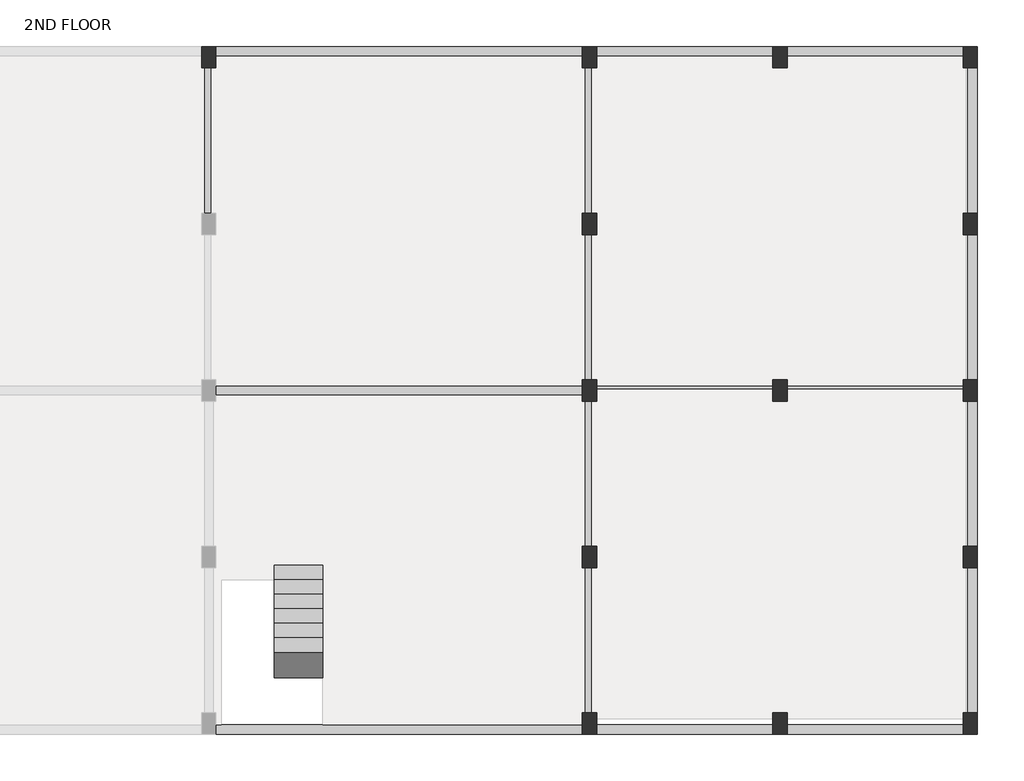
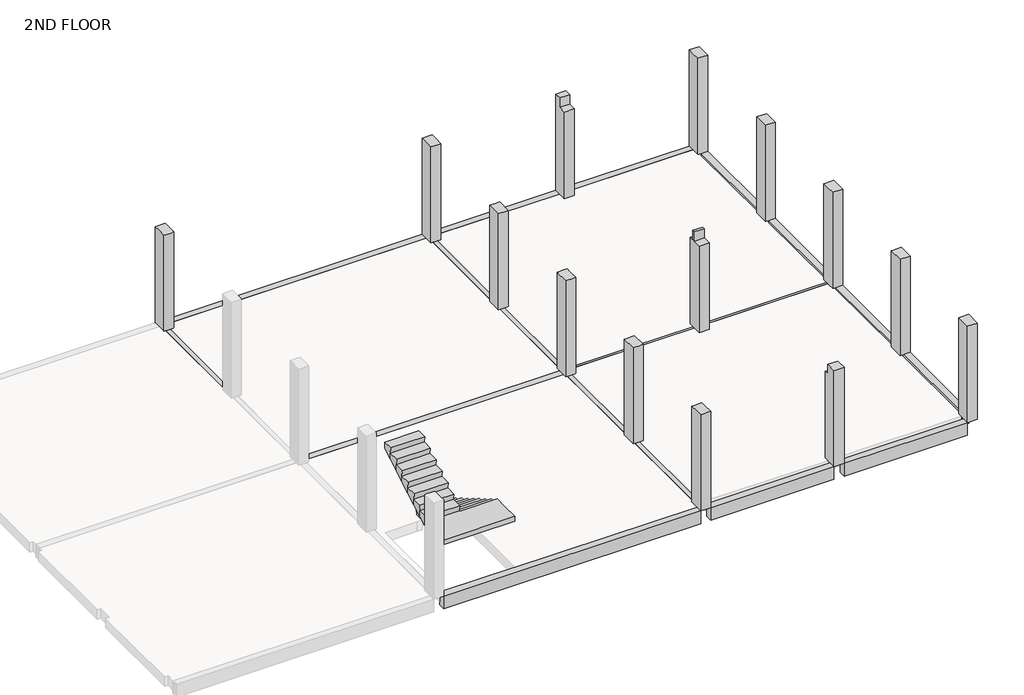
# One storey, part 2 of 2: 18 beams, 14 columns, 1 stair flight.
"""IFC4 building model written with IfcOpenShell, lengths in millimetres."""

from ifc_helpers import new_model, si_unit, frame, origin, place, context, project, spatial, polyline, outline, extrude, faceted_brep, element, save

model = new_model("IFC4")

# Units and contexts
model_context = context("Model", 3, world=origin())
ifc_project = project(units=[si_unit("LENGTHUNIT", "METRE", prefix="MILLI")], contexts=[model_context])

# Site, building, storey
site = spatial("IfcSite", under=ifc_project)
building = spatial("IfcBuilding", under=site)
storey = spatial("IfcBuildingStorey", under=building, Name="2ND FLOOR", Elevation=6096.0)

# Beams
placement = place(None, origin())
element("IfcBeam", 1, ObjectType="M_Concrete-Rectangular Beam : 200MMX400MM", at=placement, inside=storey, context=model_context, shape_type="Brep", body=[
    faceted_brep([(4019.3125983, 15797.7008557, 6096.0), (4019.3125983, 15997.7008557, 6096.0), (-3680.6874017, 15997.7008557, 6096.0), (-3680.6874017, 15797.7008557, 6096.0), (4019.3125983, 15797.7008557, 5696.0), (4019.3125983, 15797.7008557, 5796.0), (-3680.6874017, 15797.7008557, 5796.0), (-3680.6874017, 15797.7008557, 5696.0), (4019.3125983, 15997.7008557, 5696.0), (-3680.6874017, 15997.7008557, 5696.0)], [[[0, 1, 2, 3]], [[4, 5, 0, 3, 6, 7]], [[8, 4, 7, 9]], [[1, 8, 9, 2]], [[1, 0, 5, 4, 8]], [[2, 9, 7, 6, 3]]]),
])
element("IfcBeam", 2, ObjectType="M_Concrete-Rectangular Beam : 200MMX400MM", at=placement, inside=storey, context=model_context, shape_type="Brep", body=[
    faceted_brep([(8019.3125983, 15797.7008557, 6096.0), (8019.3125983, 15997.7008557, 6096.0), (4319.3125983, 15997.7008557, 6096.0), (4319.3125983, 15797.7008557, 6096.0), (8019.3125983, 15797.7008557, 5696.0), (4319.3125983, 15797.7008557, 5796.0), (4319.3125983, 15797.7008557, 5696.0), (8019.3125983, 15997.7008557, 5696.0), (4319.3125983, 15997.7008557, 5696.0)], [[[0, 1, 2, 3]], [[4, 0, 3, 5, 6]], [[7, 4, 6, 8]], [[1, 7, 8, 2]], [[2, 8, 6, 5, 3]], [[1, 0, 4, 7]]]),
])
element("IfcBeam", 3, ObjectType="M_Concrete-Rectangular Beam : 200MMX400MM", at=placement, inside=storey, context=model_context, shape_type="Brep", body=[
    faceted_brep([(12019.3125983, 15797.7008557, 6096.0), (12019.3125983, 15997.7008557, 6096.0), (8319.3125983, 15997.7008557, 6096.0), (8319.3125983, 15797.7008557, 6096.0), (12019.3125983, 15797.7008557, 5696.0), (12019.3125983, 15797.7008557, 5796.0), (8319.3125983, 15797.7008557, 5696.0), (12019.3125983, 15997.7008557, 5696.0), (8319.3125983, 15997.7008557, 5696.0)], [[[0, 1, 2, 3]], [[4, 5, 0, 3, 6]], [[7, 4, 6, 8]], [[1, 7, 8, 2]], [[2, 8, 6, 3]], [[1, 0, 5, 4, 7]]]),
])
element("IfcBeam", 4, ObjectType="M_Concrete-Rectangular Beam : 200MMX400MM", at=placement, inside=storey, context=model_context, shape_type="SweptSolid", body=[
    extrude(outline(polyline([(12319.3125983, 12497.7008557), (12119.3125983, 12497.7008557), (12119.3125983, 15547.7008557), (12319.3125983, 15547.7008557), (12319.3125983, 12497.7008557)])), frame((0.0, 0.0, 5696.0), z_axis=(0.0, 0.0, 1.0), x_axis=(1.0, 0.0, 0.0)), (0.0, 0.0, 1.0), 400.0),
])
element("IfcBeam", 5, ObjectType="M_Concrete-Rectangular Beam : 200MMX400MM", at=placement, inside=storey, context=model_context, shape_type="SweptSolid", body=[
    extrude(outline(polyline([(12319.3125983, 1997.7008557), (12119.3125983, 1997.7008557), (12119.3125983, 5047.7008557), (12319.3125983, 5047.7008557), (12319.3125983, 1997.7008557)])), frame((0.0, 0.0, 5696.0), z_axis=(0.0, 0.0, 1.0), x_axis=(1.0, 0.0, 0.0)), (0.0, 0.0, 1.0), 400.0),
])
element("IfcBeam", 6, ObjectType="M_Concrete-Rectangular Beam : 200MMX400MM", at=placement, inside=storey, context=model_context, shape_type="SweptSolid", body=[
    extrude(outline(polyline([(8319.3125983, 1547.7008557), (8319.3125983, 1747.7008557), (12019.3125983, 1747.7008557), (12019.3125983, 1547.7008557), (8319.3125983, 1547.7008557)])), frame((0.0, 0.0, 5696.0), z_axis=(0.0, 0.0, 1.0), x_axis=(1.0, 0.0, 0.0)), (0.0, 0.0, 1.0), 400.0),
])
element("IfcBeam", 7, ObjectType="M_Concrete-Rectangular Beam : 200MMX400MM", at=placement, inside=storey, context=model_context, shape_type="SweptSolid", body=[
    extrude(outline(polyline([(8019.3125983, 1747.7008557), (8019.3125983, 1547.7008557), (4319.3125983, 1547.7008557), (4319.3125983, 1747.7008557), (8019.3125983, 1747.7008557)])), frame((0.0, 0.0, 5696.0), z_axis=(0.0, 0.0, 1.0), x_axis=(1.0, 0.0, 0.0)), (0.0, 0.0, 1.0), 400.0),
])
element("IfcBeam", 8, ObjectType="M_Concrete-Rectangular Beam : 200MMX400MM", at=placement, inside=storey, context=model_context, shape_type="Brep", body=[
    faceted_brep([(-3680.6874017, 1747.7008557, 6096.0), (-3680.6874017, 1547.7008557, 6096.0), (4019.3125983, 1547.7008557, 6096.0), (4019.3125983, 1747.7008557, 6096.0), (-1437.0874017, 1747.7008557, 6096.0), (-3570.6874017, 1747.7008557, 6096.0), (-3680.6874017, 1747.7008557, 5696.0), (-3680.6874017, 1747.7008557, 5796.0), (4019.3125983, 1747.7008557, 5796.0), (4019.3125983, 1747.7008557, 5696.0), (-3680.6874017, 1547.7008557, 5696.0), (4019.3125983, 1547.7008557, 5696.0)], [[[0, 1, 2, 3, 4, 5]], [[6, 7, 0, 5, 4, 3, 8, 9]], [[10, 6, 9, 11]], [[1, 10, 11, 2]], [[1, 0, 7, 6, 10]], [[2, 11, 9, 8, 3]]]),
])
element("IfcBeam", 9, ObjectType="M_Concrete-Rectangular Beam : 200MMX400MM", at=placement, inside=storey, context=model_context, shape_type="Brep", body=[
    faceted_brep([(4019.3125983, 8872.7008557, 6096.0), (-3680.6874017, 8872.7008557, 6096.0), (-3680.6874017, 8672.7008557, 6096.0), (4019.3125983, 8672.7008557, 6096.0), (-3680.6874017, 8672.7008557, 5796.0), (-3680.6874017, 8672.7008557, 5696.0), (4019.3125983, 8672.7008557, 5696.0), (4019.3125983, 8672.7008557, 5796.0), (-3680.6874017, 8872.7008557, 5696.0), (4019.3125983, 8872.7008557, 5696.0), (4019.3125983, 8872.7008557, 5796.0), (-3680.6874017, 8872.7008557, 5796.0)], [[[0, 1, 2, 3]], [[3, 2, 4, 5, 6, 7]], [[6, 5, 8, 9]], [[1, 0, 10, 9, 8, 11]], [[8, 5, 4, 2, 1, 11]], [[0, 3, 7, 6, 9, 10]]]),
])
element("IfcBeam", 10, ObjectType="M_Concrete-Rectangular Beam : 200MMX400MM", at=placement, inside=storey, context=model_context, shape_type="Brep", body=[
    faceted_brep([(8019.3125983, 8872.7008557, 6096.0), (4319.3125983, 8872.7008557, 6096.0), (4319.3125983, 8797.7008557, 6096.0), (8019.3125983, 8797.7008557, 6096.0), (4319.3125983, 8672.7008557, 5696.0), (8019.3125983, 8672.7008557, 5696.0), (8019.3125983, 8672.7008557, 5796.0), (4319.3125983, 8672.7008557, 5796.0), (4319.3125983, 8872.7008557, 5696.0), (8019.3125983, 8872.7008557, 5696.0), (8019.3125983, 8872.7008557, 5796.0), (4319.3125983, 8872.7008557, 5796.0), (4319.3125983, 8797.7008557, 5796.0), (8019.3125983, 8797.7008557, 5796.0)], [[[0, 1, 2, 3]], [[4, 5, 6, 7]], [[5, 4, 8, 9]], [[1, 0, 10, 9, 8, 11]], [[8, 4, 7, 12, 2, 1, 11]], [[5, 9, 10, 0, 3, 13, 6]], [[13, 12, 7, 6]], [[12, 13, 3, 2]]]),
])
element("IfcBeam", 11, ObjectType="M_Concrete-Rectangular Beam : 200MMX400MM", at=placement, inside=storey, context=model_context, shape_type="Brep", body=[
    faceted_brep([(12019.3125983, 8872.7008557, 6096.0), (8319.3125983, 8872.7008557, 6096.0), (8319.3125983, 8797.7008557, 6096.0), (12019.3125983, 8797.7008557, 6096.0), (8319.3125983, 8672.7008557, 5696.0), (12019.3125983, 8672.7008557, 5696.0), (12019.3125983, 8672.7008557, 5796.0), (8319.3125983, 8672.7008557, 5796.0), (8319.3125983, 8872.7008557, 5696.0), (12019.3125983, 8872.7008557, 5696.0), (12019.3125983, 8872.7008557, 5796.0), (8319.3125983, 8872.7008557, 5796.0), (12019.3125983, 8797.7008557, 5796.0), (8319.3125983, 8797.7008557, 5796.0)], [[[0, 1, 2, 3]], [[4, 5, 6, 7]], [[5, 4, 8, 9]], [[1, 0, 10, 9, 8, 11]], [[5, 9, 10, 0, 3, 12, 6]], [[8, 4, 7, 13, 2, 1, 11]], [[12, 13, 7, 6]], [[13, 12, 3, 2]]]),
])
element("IfcBeam", 12, ObjectType="M_Concrete-Rectangular Beam : 200MMX400MM", at=placement, inside=storey, context=model_context, shape_type="SweptSolid", body=[
    extrude(outline(polyline([(12319.3125983, 5497.7008557), (12119.3125983, 5497.7008557), (12119.3125983, 8547.7008557), (12319.3125983, 8547.7008557), (12319.3125983, 5497.7008557)])), frame((0.0, 0.0, 5696.0), z_axis=(0.0, 0.0, 1.0), x_axis=(1.0, 0.0, 0.0)), (0.0, 0.0, 1.0), 400.0),
])
element("IfcBeam", 13, ObjectType="M_Concrete-Rectangular Beam : 200MMX400MM", at=placement, inside=storey, context=model_context, shape_type="SweptSolid", body=[
    extrude(outline(polyline([(12119.3125983, 12047.7008557), (12319.3125983, 12047.7008557), (12319.3125983, 8997.7008557), (12119.3125983, 8997.7008557), (12119.3125983, 12047.7008557)])), frame((0.0, 0.0, 5696.0), z_axis=(0.0, 0.0, 1.0), x_axis=(1.0, 0.0, 0.0)), (0.0, 0.0, 1.0), 400.0),
])
element("IfcBeam", 14, ObjectType="M_Concrete-Rectangular Beam : 200MMX400MM", at=placement, inside=storey, context=model_context, shape_type="Brep", body=[
    faceted_brep([(4069.3125983, 5047.7008557, 6096.0), (4069.3125983, 1997.7008557, 6096.0), (4219.3125983, 1997.7008557, 6096.0), (4219.3125983, 5047.7008557, 6096.0), (4269.3125983, 1997.7008557, 5696.0), (4269.3125983, 5047.7008557, 5696.0), (4269.3125983, 5047.7008557, 5796.0), (4269.3125983, 1997.7008557, 5796.0), (4069.3125983, 1997.7008557, 5696.0), (4069.3125983, 5047.7008557, 5696.0), (4069.3125983, 5047.7008557, 5796.0), (4069.3125983, 1997.7008557, 5796.0), (4219.3125983, 1997.7008557, 5796.0), (4219.3125983, 5047.7008557, 5796.0)], [[[0, 1, 2, 3]], [[4, 5, 6, 7]], [[5, 4, 8, 9]], [[1, 0, 10, 9, 8, 11]], [[8, 4, 7, 12, 2, 1, 11]], [[5, 9, 10, 0, 3, 13, 6]], [[13, 12, 7, 6]], [[12, 13, 3, 2]]]),
])
element("IfcBeam", 15, ObjectType="M_Concrete-Rectangular Beam : 200MMX400MM", at=placement, inside=storey, context=model_context, shape_type="Brep", body=[
    faceted_brep([(4069.3125983, 8547.7008557, 6096.0), (4069.3125983, 5497.7008557, 6096.0), (4219.3125983, 5497.7008557, 6096.0), (4219.3125983, 8547.7008557, 6096.0), (4269.3125983, 5497.7008557, 5696.0), (4269.3125983, 8547.7008557, 5696.0), (4269.3125983, 8547.7008557, 5796.0), (4269.3125983, 5497.7008557, 5796.0), (4069.3125983, 5497.7008557, 5696.0), (4069.3125983, 8547.7008557, 5696.0), (4069.3125983, 8547.7008557, 5796.0), (4069.3125983, 5497.7008557, 5796.0), (4219.3125983, 8547.7008557, 5796.0), (4219.3125983, 5497.7008557, 5796.0)], [[[0, 1, 2, 3]], [[4, 5, 6, 7]], [[5, 4, 8, 9]], [[1, 0, 10, 9, 8, 11]], [[5, 9, 10, 0, 3, 12, 6]], [[8, 4, 7, 13, 2, 1, 11]], [[12, 13, 7, 6]], [[13, 12, 3, 2]]]),
])
element("IfcBeam", 16, ObjectType="M_Concrete-Rectangular Beam : 200MMX400MM", at=placement, inside=storey, context=model_context, shape_type="Brep", body=[
    faceted_brep([(4069.3125983, 12047.7008557, 6096.0), (4069.3125983, 8997.7008557, 6096.0), (4219.3125983, 8997.7008557, 6096.0), (4219.3125983, 12047.7008557, 6096.0), (4269.3125983, 8997.7008557, 5696.0), (4269.3125983, 12047.7008557, 5696.0), (4269.3125983, 12047.7008557, 5796.0), (4269.3125983, 8997.7008557, 5796.0), (4069.3125983, 8997.7008557, 5696.0), (4069.3125983, 12047.7008557, 5696.0), (4069.3125983, 12047.7008557, 5796.0), (4069.3125983, 8997.7008557, 5796.0), (4219.3125983, 8997.7008557, 5796.0), (4219.3125983, 12047.7008557, 5796.0)], [[[0, 1, 2, 3]], [[4, 5, 6, 7]], [[5, 4, 8, 9]], [[1, 0, 10, 9, 8, 11]], [[8, 4, 7, 12, 2, 1, 11]], [[5, 9, 10, 0, 3, 13, 6]], [[13, 12, 7, 6]], [[12, 13, 3, 2]]]),
])
element("IfcBeam", 17, ObjectType="M_Concrete-Rectangular Beam : 200MMX400MM", at=placement, inside=storey, context=model_context, shape_type="Brep", body=[
    faceted_brep([(4069.3125983, 15547.7008557, 6096.0), (4069.3125983, 12497.7008557, 6096.0), (4219.3125983, 12497.7008557, 6096.0), (4219.3125983, 15547.7008557, 6096.0), (4269.3125983, 12497.7008557, 5696.0), (4269.3125983, 15547.7008557, 5696.0), (4269.3125983, 15547.7008557, 5796.0), (4269.3125983, 12497.7008557, 5796.0), (4069.3125983, 12497.7008557, 5696.0), (4069.3125983, 15547.7008557, 5696.0), (4069.3125983, 15547.7008557, 5796.0), (4069.3125983, 12497.7008557, 5796.0), (4219.3125983, 15547.7008557, 5796.0), (4219.3125983, 12497.7008557, 5796.0)], [[[0, 1, 2, 3]], [[4, 5, 6, 7]], [[5, 4, 8, 9]], [[1, 0, 10, 9, 8, 11]], [[5, 9, 10, 0, 3, 12, 6]], [[8, 4, 7, 13, 2, 1, 11]], [[12, 13, 7, 6]], [[13, 12, 3, 2]]]),
])
element("IfcBeam", 18, ObjectType="M_Concrete-Rectangular Beam : 200MMX400MM", at=placement, inside=storey, context=model_context, shape_type="Brep", body=[
    faceted_brep([(-3930.6874017, 15547.7008557, 6096.0), (-3930.6874017, 12497.7008557, 6096.0), (-3780.6874017, 12497.7008557, 6096.0), (-3780.6874017, 15547.7008557, 6096.0), (-3730.6874017, 12497.7008557, 5696.0), (-3730.6874017, 15547.7008557, 5696.0), (-3730.6874017, 15547.7008557, 5796.0), (-3730.6874017, 12497.7008557, 5796.0), (-3930.6874017, 12497.7008557, 5696.0), (-3930.6874017, 15547.7008557, 5696.0), (-3930.6874017, 15547.7008557, 5796.0), (-3930.6874017, 12497.7008557, 5796.0), (-3780.6874017, 15547.7008557, 5796.0), (-3780.6874017, 12497.7008557, 5796.0)], [[[0, 1, 2, 3]], [[4, 5, 6, 7]], [[5, 4, 8, 9]], [[1, 0, 10, 9, 8, 11]], [[5, 9, 10, 0, 3, 12, 6]], [[8, 4, 7, 13, 2, 1, 11]], [[12, 13, 7, 6]], [[13, 12, 3, 2]]]),
])

# Columns
element("IfcColumn", 19, ObjectType="M_Concrete-Rectangular-Column : 300 x 450mm", at=placement, inside=storey, context=model_context, shape_type="Brep", body=[
    faceted_brep([(-3680.6874017, 15997.7008557, 6096.0), (-3680.6874017, 15547.7008557, 6096.0), (-3980.6874017, 15547.7008557, 6096.0), (-3980.6874017, 15997.7008557, 6096.0), (-3680.6874017, 15997.7008557, 9144.0), (-3680.6874017, 15797.7008557, 9144.0), (-3680.6874017, 15547.7008557, 9144.0), (-3680.6874017, 15547.7008557, 8844.0), (-3780.6874017, 15547.7008557, 9144.0), (-3930.6874017, 15547.7008557, 9144.0), (-3980.6874017, 15547.7008557, 9144.0), (-3980.6874017, 15547.7008557, 8844.0), (-3980.6874017, 15797.7008557, 9144.0), (-3980.6874017, 15997.7008557, 9144.0)], [[[0, 1, 2, 3]], [[1, 0, 4, 5, 6, 7]], [[2, 1, 7, 6, 8, 9, 10, 11]], [[3, 2, 11, 10, 12, 13]], [[0, 3, 13, 4]], [[4, 13, 12, 10, 9, 8, 6, 5]]]),
])
element("IfcColumn", 20, ObjectType="M_Concrete-Rectangular-Column : 300 x 450mm", at=placement, inside=storey, context=model_context, shape_type="Brep", body=[
    faceted_brep([(4319.3125983, 15997.7008557, 6096.0), (4319.3125983, 15547.7008557, 6096.0), (4019.3125983, 15547.7008557, 6096.0), (4019.3125983, 15997.7008557, 6096.0), (4319.3125983, 15997.7008557, 9144.0), (4319.3125983, 15797.7008557, 9144.0), (4319.3125983, 15547.7008557, 9144.0), (4319.3125983, 15547.7008557, 8844.0), (4219.3125983, 15547.7008557, 9144.0), (4069.3125983, 15547.7008557, 9144.0), (4019.3125983, 15547.7008557, 9144.0), (4019.3125983, 15547.7008557, 8844.0), (4019.3125983, 15797.7008557, 9144.0), (4019.3125983, 15997.7008557, 9144.0)], [[[0, 1, 2, 3]], [[1, 0, 4, 5, 6, 7]], [[2, 1, 7, 6, 8, 9, 10, 11]], [[3, 2, 11, 10, 12, 13]], [[0, 3, 13, 4]], [[4, 13, 12, 10, 9, 8, 6, 5]]]),
])
element("IfcColumn", 21, ObjectType="M_Concrete-Rectangular-Column : 300 x 450mm", at=placement, inside=storey, context=model_context, shape_type="Brep", body=[
    faceted_brep([(4319.3125983, 8997.7008557, 6096.0), (4319.3125983, 8547.7008557, 6096.0), (4019.3125983, 8547.7008557, 6096.0), (4019.3125983, 8997.7008557, 6096.0), (4319.3125983, 8997.7008557, 8844.0), (4319.3125983, 8997.7008557, 9144.0), (4319.3125983, 8872.7008557, 9144.0), (4319.3125983, 8797.7008557, 9144.0), (4319.3125983, 8547.7008557, 9144.0), (4319.3125983, 8547.7008557, 8844.0), (4219.3125983, 8547.7008557, 9144.0), (4069.3125983, 8547.7008557, 9144.0), (4019.3125983, 8547.7008557, 9144.0), (4019.3125983, 8547.7008557, 8844.0), (4019.3125983, 8672.7008557, 9144.0), (4019.3125983, 8872.7008557, 9144.0), (4019.3125983, 8997.7008557, 9144.0), (4019.3125983, 8997.7008557, 8844.0), (4069.3125983, 8997.7008557, 9144.0), (4219.3125983, 8997.7008557, 9144.0)], [[[0, 1, 2, 3]], [[1, 0, 4, 5, 6, 7, 8, 9]], [[2, 1, 9, 8, 10, 11, 12, 13]], [[3, 2, 13, 12, 14, 15, 16, 17]], [[0, 3, 17, 16, 18, 19, 5, 4]], [[18, 16, 15, 14, 12, 11, 10, 8, 7, 6, 5, 19]]]),
])
element("IfcColumn", 22, ObjectType="M_Concrete-Rectangular-Column : 300 x 450mm", at=placement, inside=storey, context=model_context, shape_type="Brep", body=[
    faceted_brep([(4319.3125983, 1997.7008557, 6096.0), (4319.3125983, 1547.7008557, 6096.0), (4019.3125983, 1547.7008557, 6096.0), (4019.3125983, 1997.7008557, 6096.0), (4319.3125983, 1997.7008557, 8844.0), (4319.3125983, 1997.7008557, 9144.0), (4319.3125983, 1872.7008557, 9144.0), (4319.3125983, 1547.7008557, 9144.0), (4019.3125983, 1547.7008557, 9144.0), (4019.3125983, 1747.7008557, 9144.0), (4019.3125983, 1997.7008557, 9144.0), (4019.3125983, 1997.7008557, 8844.0), (4069.3125983, 1997.7008557, 9144.0), (4219.3125983, 1997.7008557, 9144.0)], [[[0, 1, 2, 3]], [[1, 0, 4, 5, 6, 7]], [[2, 1, 7, 8]], [[3, 2, 8, 9, 10, 11]], [[0, 3, 11, 10, 12, 13, 5, 4]], [[8, 7, 6, 5, 13, 12, 10, 9]]]),
])
element("IfcColumn", 23, ObjectType="M_Concrete-Rectangular-Column : 300 x 450mm", at=placement, inside=storey, context=model_context, shape_type="SweptSolid", body=[
    extrude(outline(polyline([(15997.7008557, 6096.0), (15547.7008557, 6096.0), (15547.7008557, 8844.0), (15797.7008557, 8844.0), (15797.7008557, 9144.0), (15997.7008557, 9144.0), (15997.7008557, 6096.0)])), frame((8019.3125983, 0.0, 0.0), z_axis=(1.0, 0.0, 0.0), x_axis=(0.0, 1.0, 0.0)), (0.0, 0.0, 1.0), 300.0),
])
element("IfcColumn", 24, ObjectType="M_Concrete-Rectangular-Column : 300 x 450mm", at=placement, inside=storey, context=model_context, shape_type="SweptSolid", body=[
    extrude(outline(polyline([(1997.7008557, 6096.0), (1547.7008557, 6096.0), (1547.7008557, 9144.0), (1872.7008557, 9144.0), (1872.7008557, 8844.0), (1997.7008557, 8844.0), (1997.7008557, 6096.0)])), frame((8019.3125983, 0.0, 0.0), z_axis=(1.0, 0.0, 0.0), x_axis=(0.0, 1.0, 0.0)), (0.0, 0.0, 1.0), 300.0),
])
element("IfcColumn", 25, ObjectType="M_Concrete-Rectangular-Column : 300 x 450mm", at=placement, inside=storey, context=model_context, shape_type="Brep", body=[
    faceted_brep([(12319.3125983, 12497.7008557, 6096.0), (12319.3125983, 12047.7008557, 6096.0), (12019.3125983, 12047.7008557, 6096.0), (12019.3125983, 12497.7008557, 6096.0), (12319.3125983, 12497.7008557, 9144.0), (12319.3125983, 12047.7008557, 9144.0), (12069.3125983, 12047.7008557, 9144.0), (12019.3125983, 12047.7008557, 9144.0), (12019.3125983, 12047.7008557, 8844.0), (12019.3125983, 12497.7008557, 9144.0), (12019.3125983, 12497.7008557, 8844.0), (12069.3125983, 12497.7008557, 9144.0)], [[[0, 1, 2, 3]], [[1, 0, 4, 5]], [[2, 1, 5, 6, 7, 8]], [[3, 2, 8, 7, 9, 10]], [[0, 3, 10, 9, 11, 4]], [[5, 4, 11, 9, 7, 6]]]),
])
element("IfcColumn", 26, ObjectType="M_Concrete-Rectangular-Column : 300 x 450mm", at=placement, inside=storey, context=model_context, shape_type="Brep", body=[
    faceted_brep([(12319.3125983, 5497.7008557, 6096.0), (12319.3125983, 5047.7008557, 6096.0), (12019.3125983, 5047.7008557, 6096.0), (12019.3125983, 5497.7008557, 6096.0), (12319.3125983, 5497.7008557, 9144.0), (12319.3125983, 5047.7008557, 9144.0), (12069.3125983, 5047.7008557, 9144.0), (12019.3125983, 5047.7008557, 9144.0), (12019.3125983, 5047.7008557, 8844.0), (12019.3125983, 5497.7008557, 9144.0), (12019.3125983, 5497.7008557, 8844.0), (12069.3125983, 5497.7008557, 9144.0)], [[[0, 1, 2, 3]], [[1, 0, 4, 5]], [[2, 1, 5, 6, 7, 8]], [[3, 2, 8, 7, 9, 10]], [[0, 3, 10, 9, 11, 4]], [[5, 4, 11, 9, 7, 6]]]),
])
element("IfcColumn", 27, ObjectType="M_Concrete-Rectangular-Column : 300 x 450mm", at=placement, inside=storey, context=model_context, shape_type="Brep", body=[
    faceted_brep([(12319.3125983, 15997.7008557, 6096.0), (12319.3125983, 15547.7008557, 6096.0), (12019.3125983, 15547.7008557, 6096.0), (12019.3125983, 15997.7008557, 6096.0), (12319.3125983, 15997.7008557, 9144.0), (12319.3125983, 15547.7008557, 9144.0), (12069.3125983, 15547.7008557, 9144.0), (12019.3125983, 15547.7008557, 9144.0), (12019.3125983, 15547.7008557, 8844.0), (12019.3125983, 15797.7008557, 9144.0), (12019.3125983, 15997.7008557, 9144.0)], [[[0, 1, 2, 3]], [[1, 0, 4, 5]], [[2, 1, 5, 6, 7, 8]], [[3, 2, 8, 7, 9, 10]], [[0, 3, 10, 4]], [[5, 4, 10, 9, 7, 6]]]),
])
element("IfcColumn", 28, ObjectType="M_Concrete-Rectangular-Column : 300 x 450mm", at=placement, inside=storey, context=model_context, shape_type="Brep", body=[
    faceted_brep([(12319.3125983, 1997.7008557, 6096.0), (12319.3125983, 1547.7008557, 6096.0), (12019.3125983, 1547.7008557, 6096.0), (12019.3125983, 1997.7008557, 6096.0), (12319.3125983, 1997.7008557, 9144.0), (12319.3125983, 1547.7008557, 9144.0), (12019.3125983, 1547.7008557, 9144.0), (12019.3125983, 1872.7008557, 9144.0), (12019.3125983, 1997.7008557, 9144.0), (12019.3125983, 1997.7008557, 8844.0), (12069.3125983, 1997.7008557, 9144.0)], [[[0, 1, 2, 3]], [[1, 0, 4, 5]], [[2, 1, 5, 6]], [[3, 2, 6, 7, 8, 9]], [[0, 3, 9, 8, 10, 4]], [[5, 4, 10, 8, 7, 6]]]),
])
element("IfcColumn", 29, ObjectType="M_Concrete-Rectangular-Column : 300 x 450mm", at=placement, inside=storey, context=model_context, shape_type="Brep", body=[
    faceted_brep([(12319.3125983, 8997.7008557, 6096.0), (12319.3125983, 8547.7008557, 6096.0), (12019.3125983, 8547.7008557, 6096.0), (12019.3125983, 8997.7008557, 6096.0), (12319.3125983, 8997.7008557, 9144.0), (12319.3125983, 8547.7008557, 9144.0), (12069.3125983, 8547.7008557, 9144.0), (12019.3125983, 8547.7008557, 9144.0), (12019.3125983, 8547.7008557, 8844.0), (12019.3125983, 8797.7008557, 9144.0), (12019.3125983, 8872.7008557, 9144.0), (12019.3125983, 8997.7008557, 9144.0), (12019.3125983, 8997.7008557, 8844.0), (12069.3125983, 8997.7008557, 9144.0)], [[[0, 1, 2, 3]], [[1, 0, 4, 5]], [[2, 1, 5, 6, 7, 8]], [[3, 2, 8, 7, 9, 10, 11, 12]], [[0, 3, 12, 11, 13, 4]], [[5, 4, 13, 11, 10, 9, 7, 6]]]),
])
element("IfcColumn", 30, ObjectType="M_Concrete-Rectangular-Column : 300 x 450mm", at=placement, inside=storey, context=model_context, shape_type="Brep", body=[
    faceted_brep([(8319.3125983, 8997.7008557, 6096.0), (8319.3125983, 8547.7008557, 6096.0), (8019.3125983, 8547.7008557, 6096.0), (8019.3125983, 8997.7008557, 6096.0), (8319.3125983, 8997.7008557, 8844.0), (8319.3125983, 8872.7008557, 8844.0), (8319.3125983, 8872.7008557, 9144.0), (8319.3125983, 8797.7008557, 9144.0), (8319.3125983, 8797.7008557, 8844.0), (8319.3125983, 8547.7008557, 8844.0), (8019.3125983, 8547.7008557, 8844.0), (8019.3125983, 8672.7008557, 8844.0), (8019.3125983, 8797.7008557, 8844.0), (8019.3125983, 8797.7008557, 9144.0), (8019.3125983, 8872.7008557, 9144.0), (8019.3125983, 8872.7008557, 8844.0), (8019.3125983, 8997.7008557, 8844.0)], [[[0, 1, 2, 3]], [[1, 0, 4, 5, 6, 7, 8, 9]], [[2, 1, 9, 10]], [[3, 2, 10, 11, 12, 13, 14, 15, 16]], [[0, 3, 16, 4]], [[14, 13, 7, 6]], [[8, 12, 11, 10, 9]], [[5, 15, 14, 6]], [[12, 8, 7, 13]], [[15, 5, 4, 16]]]),
])
element("IfcColumn", 31, ObjectType="M_Concrete-Rectangular-Column : 300 x 450mm", at=placement, inside=storey, context=model_context, shape_type="Brep", body=[
    faceted_brep([(4319.3125983, 12497.7008557, 6096.0), (4319.3125983, 12047.7008557, 6096.0), (4019.3125983, 12047.7008557, 6096.0), (4019.3125983, 12497.7008557, 6096.0), (4319.3125983, 12497.7008557, 8844.0), (4319.3125983, 12497.7008557, 9144.0), (4319.3125983, 12047.7008557, 9144.0), (4319.3125983, 12047.7008557, 8844.0), (4219.3125983, 12047.7008557, 9144.0), (4069.3125983, 12047.7008557, 9144.0), (4019.3125983, 12047.7008557, 9144.0), (4019.3125983, 12047.7008557, 8844.0), (4019.3125983, 12497.7008557, 9144.0), (4019.3125983, 12497.7008557, 8844.0), (4069.3125983, 12497.7008557, 9144.0), (4219.3125983, 12497.7008557, 9144.0)], [[[0, 1, 2, 3]], [[1, 0, 4, 5, 6, 7]], [[2, 1, 7, 6, 8, 9, 10, 11]], [[3, 2, 11, 10, 12, 13]], [[0, 3, 13, 12, 14, 15, 5, 4]], [[6, 5, 15, 14, 12, 10, 9, 8]]]),
])
element("IfcColumn", 32, ObjectType="M_Concrete-Rectangular-Column : 300 x 450mm", at=placement, inside=storey, context=model_context, shape_type="Brep", body=[
    faceted_brep([(4319.3125983, 5497.7008557, 6096.0), (4319.3125983, 5047.7008557, 6096.0), (4019.3125983, 5047.7008557, 6096.0), (4019.3125983, 5497.7008557, 6096.0), (4319.3125983, 5497.7008557, 8844.0), (4319.3125983, 5497.7008557, 9144.0), (4319.3125983, 5047.7008557, 9144.0), (4319.3125983, 5047.7008557, 8844.0), (4219.3125983, 5047.7008557, 9144.0), (4069.3125983, 5047.7008557, 9144.0), (4019.3125983, 5047.7008557, 9144.0), (4019.3125983, 5047.7008557, 8844.0), (4019.3125983, 5497.7008557, 9144.0), (4019.3125983, 5497.7008557, 8844.0), (4069.3125983, 5497.7008557, 9144.0), (4219.3125983, 5497.7008557, 9144.0)], [[[0, 1, 2, 3]], [[1, 0, 4, 5, 6, 7]], [[2, 1, 7, 6, 8, 9, 10, 11]], [[3, 2, 11, 10, 12, 13]], [[0, 3, 13, 12, 14, 15, 5, 4]], [[6, 5, 15, 14, 12, 10, 9, 8]]]),
])

# Stair flight
element("IfcStairFlight", 33, ObjectType="25 mm Nosing", at=placement, inside=storey, context=model_context, shape_type="Brep", body=[
    faceted_brep([(-1437.0874017, 5100.5008557, 6275.2941176), (-2453.0874017, 5100.5008557, 6275.2941176), (-2453.0874017, 4770.7008557, 6275.2941176), (-1437.0874017, 4770.7008557, 6275.2941176), (-1437.0874017, 4770.7008557, 6101.2669154), (-1437.0874017, 4779.6546118, 6096.0), (-1437.0874017, 5075.5008557, 6096.0), (-2453.0874017, 5075.5008557, 6096.0), (-2453.0874017, 4779.6546118, 6096.0), (-2453.0874017, 4770.7008557, 6101.2669154), (-1437.0874017, 4795.7008557, 6454.5882353), (-2453.0874017, 4795.7008557, 6454.5882353), (-2453.0874017, 4465.9008557, 6454.5882353), (-1437.0874017, 4465.9008557, 6454.5882353), (-1437.0874017, 4465.9008557, 6280.561033), (-2453.0874017, 4465.9008557, 6280.561033), (-1437.0874017, 4490.9008557, 6633.8823529), (-2453.0874017, 4490.9008557, 6633.8823529), (-2453.0874017, 4161.1008557, 6633.8823529), (-1437.0874017, 4161.1008557, 6633.8823529), (-1437.0874017, 4161.1008557, 6459.8551507), (-2453.0874017, 4161.1008557, 6459.8551507), (-1437.0874017, 4186.1008557, 6813.1764706), (-2453.0874017, 4186.1008557, 6813.1764706), (-2453.0874017, 3856.3008557, 6813.1764706), (-1437.0874017, 3856.3008557, 6813.1764706), (-1437.0874017, 3856.3008557, 6639.1492683), (-2453.0874017, 3856.3008557, 6639.1492683), (-1437.0874017, 3881.3008557, 6992.4705882), (-2453.0874017, 3881.3008557, 6992.4705882), (-2453.0874017, 3551.5008557, 6992.4705882), (-1437.0874017, 3551.5008557, 6992.4705882), (-1437.0874017, 3551.5008557, 6818.443386), (-2453.0874017, 3551.5008557, 6818.443386), (-1437.0874017, 3576.5008557, 7171.7647059), (-2453.0874017, 3576.5008557, 7171.7647059), (-2453.0874017, 3246.7008557, 7171.7647059), (-1437.0874017, 3246.7008557, 7171.7647059), (-1437.0874017, 3246.7008557, 6997.7375036), (-2453.0874017, 3246.7008557, 6997.7375036), (-1437.0874017, 3271.7008557, 7351.0588235), (-2453.0874017, 3271.7008557, 7351.0588235), (-2453.0874017, 2941.9008557, 7351.0588235), (-1437.0874017, 2941.9008557, 7351.0588235), (-1437.0874017, 2941.9008557, 7177.0316213), (-2453.0874017, 2941.9008557, 7177.0316213), (-1437.0874017, 2966.9008557, 7530.3529412), (-2453.0874017, 2966.9008557, 7530.3529412), (-2453.0874017, 2637.1008557, 7530.3529412), (-1437.0874017, 2637.1008557, 7530.3529412), (-1437.0874017, 2637.1008557, 7356.3257389), (-2453.0874017, 2291.4546118, 7559.6470588), (-2453.0874017, 2641.1855014, 7559.6470588), (-3570.6874017, 2687.1008557, 7709.6470588), (-3570.6874017, 1747.7008557, 7709.6470588), (-1437.0874017, 1747.7008557, 7709.6470588), (-1437.0874017, 2291.4546118, 7709.6470588), (-1437.0874017, 2662.1008557, 7709.6470588), (-2453.0874017, 2662.1008557, 7709.6470588), (-2554.6874017, 2662.1008557, 7709.6470588), (-2554.6874017, 2687.1008557, 7709.6470588), (-3570.6874017, 2687.1008557, 7559.6470588), (-3570.6874017, 1747.7008557, 7559.6470588), (-1437.0874017, 1747.7008557, 7559.6470588), (-1437.0874017, 2291.4546118, 7559.6470588), (-2453.0874017, 2662.1008557, 7559.6470588), (-2554.6874017, 2662.1008557, 7559.6470588), (-2554.6874017, 2687.1008557, 7559.6470588), (-3570.6874017, 2662.1008557, 7888.9411765), (-2554.6874017, 2662.1008557, 7888.9411765), (-2554.6874017, 2727.9470995, 7888.9411765), (-2554.6874017, 2991.9008557, 7888.9411765), (-3570.6874017, 2991.9008557, 7888.9411765), (-3570.6874017, 2727.9470995, 7888.9411765), (-3570.6874017, 2991.9008557, 7714.9139742), (-3570.6874017, 2727.9470995, 7559.6470588), (-2554.6874017, 2727.9470995, 7559.6470588), (-2554.6874017, 2991.9008557, 7714.9139742), (-3570.6874017, 2966.9008557, 8068.2352941), (-2554.6874017, 2966.9008557, 8068.2352941), (-2554.6874017, 3296.7008557, 8068.2352941), (-3570.6874017, 3296.7008557, 8068.2352941), (-3570.6874017, 3296.7008557, 7894.2080919), (-2554.6874017, 3296.7008557, 7894.2080919), (-3570.6874017, 3271.7008557, 8247.5294118), (-2554.6874017, 3271.7008557, 8247.5294118), (-2554.6874017, 3601.5008557, 8247.5294118), (-3570.6874017, 3601.5008557, 8247.5294118), (-3570.6874017, 3601.5008557, 8073.5022095), (-2554.6874017, 3601.5008557, 8073.5022095), (-3570.6874017, 3576.5008557, 8426.8235294), (-2554.6874017, 3576.5008557, 8426.8235294), (-2554.6874017, 3906.3008557, 8426.8235294), (-3570.6874017, 3906.3008557, 8426.8235294), (-3570.6874017, 3906.3008557, 8252.7963271), (-2554.6874017, 3906.3008557, 8252.7963271), (-3570.6874017, 3881.3008557, 8606.1176471), (-2554.6874017, 3881.3008557, 8606.1176471), (-2554.6874017, 4211.1008557, 8606.1176471), (-3570.6874017, 4211.1008557, 8606.1176471), (-3570.6874017, 4211.1008557, 8432.0904448), (-2554.6874017, 4211.1008557, 8432.0904448), (-3570.6874017, 4186.1008557, 8785.4117647), (-2554.6874017, 4186.1008557, 8785.4117647), (-2554.6874017, 4515.9008557, 8785.4117647), (-3570.6874017, 4515.9008557, 8785.4117647), (-3570.6874017, 4515.9008557, 8611.3845624), (-2554.6874017, 4515.9008557, 8611.3845624), (-3570.6874017, 4490.9008557, 8964.7058824), (-2554.6874017, 4490.9008557, 8964.7058824), (-2554.6874017, 4795.7008557, 8964.7058824), (-3570.6874017, 4795.7008557, 8964.7058824), (-3570.6874017, 4795.7008557, 8775.9727977), (-2554.6874017, 4795.7008557, 8775.9727977)], [[[0, 1, 2, 3]], [[0, 3, 4, 5, 6]], [[2, 1, 7, 8, 9]], [[10, 11, 12, 13]], [[10, 13, 14, 4, 3]], [[12, 11, 2, 9, 15]], [[16, 17, 18, 19]], [[16, 19, 20, 14, 13]], [[18, 17, 12, 15, 21]], [[22, 23, 24, 25]], [[22, 25, 26, 20, 19]], [[24, 23, 18, 21, 27]], [[28, 29, 30, 31]], [[28, 31, 32, 26, 25]], [[30, 29, 24, 27, 33]], [[34, 35, 36, 37]], [[34, 37, 38, 32, 31]], [[36, 35, 30, 33, 39]], [[40, 41, 42, 43]], [[40, 43, 44, 38, 37]], [[42, 41, 36, 39, 45]], [[46, 47, 48, 49]], [[46, 49, 50, 44, 43]], [[47, 42, 45, 51, 52, 48]], [[53, 54, 55, 56, 57, 58, 59, 60]], [[54, 53, 61, 62]], [[55, 54, 62, 63]], [[49, 57, 56, 55, 63, 64, 50]], [[58, 52, 65]], [[59, 58, 65, 66]], [[60, 59, 66, 67]], [[68, 69, 70, 71, 72, 73]], [[53, 68, 73, 72, 74, 75, 61]], [[69, 60, 67, 76, 77, 71, 70]], [[78, 79, 80, 81]], [[78, 81, 82, 74, 72]], [[80, 79, 71, 77, 83]], [[84, 85, 86, 87]], [[84, 87, 88, 82, 81]], [[86, 85, 80, 83, 89]], [[90, 91, 92, 93]], [[90, 93, 94, 88, 87]], [[92, 91, 86, 89, 95]], [[96, 97, 98, 99]], [[96, 99, 100, 94, 93]], [[98, 97, 92, 95, 101]], [[102, 103, 104, 105]], [[102, 105, 106, 100, 99]], [[104, 103, 98, 101, 107]], [[1, 0, 6, 7]], [[3, 2, 11, 10]], [[13, 12, 17, 16]], [[19, 18, 23, 22]], [[25, 24, 29, 28]], [[31, 30, 35, 34]], [[37, 36, 41, 40]], [[43, 42, 47, 46]], [[49, 48, 52, 58, 57]], [[53, 60, 69, 68]], [[72, 71, 79, 78]], [[81, 80, 85, 84]], [[87, 86, 91, 90]], [[93, 92, 97, 96]], [[99, 98, 103, 102]], [[108, 109, 110, 111]], [[108, 111, 112, 106, 105]], [[110, 109, 104, 107, 113]], [[111, 110, 113, 112]], [[105, 104, 109, 108]], [[7, 6, 5, 8]], [[64, 51, 45, 39, 33, 27, 21, 15, 9, 8, 5, 4, 14, 20, 26, 32, 38, 44, 50]], [[51, 64, 63, 62, 61, 75, 76, 67, 66, 65, 52]], [[76, 75, 74, 82, 88, 94, 100, 106, 112, 113, 107, 101, 95, 89, 83, 77]]]),
])

save(model, "model.ifc")

# Revit data of these elements
# Type "M_Concrete-Rectangular Beam : 200MMX400MM"
#   Length [instance default] = 5' - 0"
#   b = 0' - 7.87402"
#   h = 1' - 3.74803"
#   Structural Material [instance default] = Concrete, Cast-in-Place gray
#   Assembly Code = ""
# Type "M_Concrete-Rectangular-Column : 300 x 450mm"
#   b = 0' - 11.81102"
#   h = 1' - 5.71654"
#   Structural Material [instance default] = Concrete, Cast-in-Place gray
# Elements 1, 2, 3, 4, 5, 6, 7, 8, 9, 10, 11, 12, 13, 14, 15, 16, 17, 18 (IfcBeam, "M_Concrete-Rectangular Beam : 200MMX400MM")
#   Structural Material = Concrete, Cast-in-Place gray
#   Phase Created = New Construction
#   Materials on its faces: "Concrete, Cast-in-Place gray"
# Elements 19, 20, 21, 22, 23, 24, 25, 26, 27, 28, 29, 30, 31, 32 (IfcColumn, "M_Concrete-Rectangular-Column : 300 x 450mm")
#   Structural Material = Concrete, Cast-in-Place gray
#   Phase Created = New Construction
#   Materials on its faces: "Concrete, Cast-in-Place gray"
# Element 33 (IfcStairFlight, "25 mm Nosing")
#   Phase Created = New Construction
#   Materials on its faces: "Concrete, Cast In Situ"
# Materials
#   "Concrete, Cast-in-Place gray": class "Concrete", colour RGB 192 192 192, transparency 0, Description = "Cast-in-place concrete", Cost = 0
#   "Concrete, Cast In Situ": class "Concrete", colour RGB 192 192 192, transparency 0, Description = "physical material", Cost = 0
